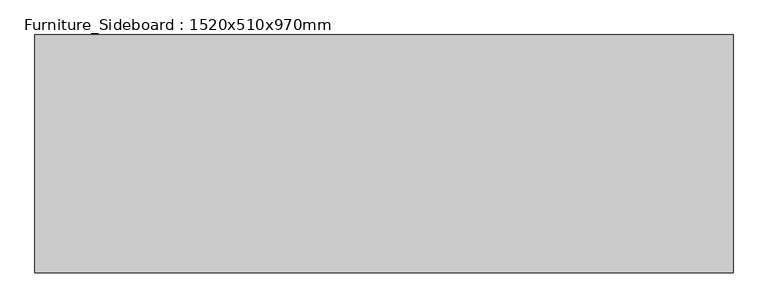
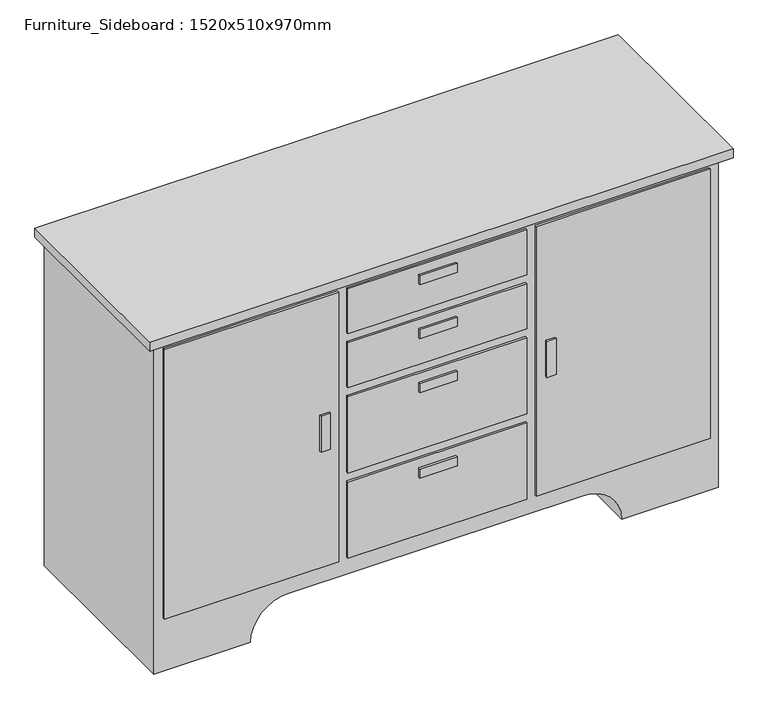
"""IFC4 building model written with IfcOpenShell, lengths in millimetres: furniture geometry, Furniture_Sideboard : 1520x510x970mm."""

from ifc_helpers import new_model, si_unit, point, frame, frame_2d, origin, place, context, project, spatial, polyline, circle_curve, trimmed, segment, composite_curve, outline, extrude, source, transform, mapped, element, save


def furniture_sideboard_1520x510x970mm_787d3fa7(model_context):
    return source(origin(), model_context, "Body", "SweptSolid", [
        extrude(outline(composite_curve([segment(polyline([(0.3974948, 465.4067402), (944.9401786, 465.4067402), (944.9401786, -1054.5932598), (0.3401786, -1054.5932598), (0.3401786, -794.7676781)]), True, "CONTINUOUS"), segment(trimmed(circle_curve(frame_2d((0.3401786, -691.2410879)), 103.5265902), [point((0.3401786, -794.7676781))], [point((103.8667688, -691.2410879))], True, "CARTESIAN"), True, "CONTINUOUS"), segment(polyline([(103.8667688, -691.2410879), (103.8667688, 102.4734638)]), True, "CONTINUOUS"), segment(trimmed(circle_curve(frame_2d((0.3974948, 102.4734638)), 103.469274), [point((103.8667688, 102.4734638))], [point((0.3974948, 205.9427378))], True, "CARTESIAN"), True, "CONTINUOUS"), segment(polyline([(0.3974948, 205.9427378), (0.3974948, 465.4067402)]), True, "CONTINUOUS")], self_intersect=False)), frame((0.0, -618.1629541, 0.0), z_axis=(0.0, 1.0, 0.0), x_axis=(0.0, 0.0, 1.0)), (0.0, 0.0, 1.0), 510.0),
        extrude(outline(polyline([(490.8067402, -643.5629541), (-1079.9932598, -643.5629541), (-1079.9932598, -108.1629541), (490.8067402, -108.1629541), (490.8067402, -643.5629541)])), frame((0.0, 0.0, 944.9401786), z_axis=(0.0, 0.0, 1.0), x_axis=(1.0, 0.0, 0.0)), (0.0, 0.0, 1.0), 25.4),
        extrude(outline(polyline([(-560.6265932, -624.5129541), (-1029.1932598, -624.5129541), (-1029.1932598, -618.1629541), (-560.6265932, -618.1629541), (-560.6265932, -624.5129541)])), frame((0.0, 0.0, 152.4), z_axis=(0.0, 0.0, 1.0), x_axis=(1.0, 0.0, 0.0)), (0.0, 0.0, 1.0), 767.1401786),
        extrude(outline(polyline([(440.0067402, -624.5129541), (-28.5599265, -624.5129541), (-28.5599265, -618.1629541), (440.0067402, -618.1629541), (440.0067402, -624.5129541)])), frame((0.0, 0.0, 152.4), z_axis=(0.0, 0.0, 1.0), x_axis=(1.0, 0.0, 0.0)), (0.0, 0.0, 1.0), 767.1401786),
        extrude(outline(polyline([(-53.9599265, -624.5129541), (-535.2265932, -624.5129541), (-535.2265932, -618.1629541), (-53.9599265, -618.1629541), (-53.9599265, -624.5129541)])), frame((0.0, 0.0, 791.5121429), z_axis=(0.0, 0.0, 1.0), x_axis=(1.0, 0.0, 0.0)), (0.0, 0.0, 1.0), 128.0280357),
        extrude(outline(polyline([(-53.9599265, -624.5129541), (-535.2265932, -624.5129541), (-535.2265932, -618.1629541), (-53.9599265, -618.1629541), (-53.9599265, -624.5129541)])), frame((0.0, 0.0, 638.0841071), z_axis=(0.0, 0.0, 1.0), x_axis=(1.0, 0.0, 0.0)), (0.0, 0.0, 1.0), 128.0280357),
        extrude(outline(polyline([(-53.9599265, -624.5129541), (-535.2265932, -624.5129541), (-535.2265932, -618.1629541), (-53.9599265, -618.1629541), (-53.9599265, -624.5129541)])), frame((0.0, 0.0, 395.2420536), z_axis=(0.0, 0.0, 1.0), x_axis=(1.0, 0.0, 0.0)), (0.0, 0.0, 1.0), 217.4420536),
        extrude(outline(polyline([(-53.9599265, -624.5129541), (-535.2265932, -624.5129541), (-535.2265932, -618.1629541), (-53.9599265, -618.1629541), (-53.9599265, -624.5129541)])), frame((0.0, 0.0, 152.4), z_axis=(0.0, 0.0, 1.0), x_axis=(1.0, 0.0, 0.0)), (0.0, 0.0, 1.0), 217.4420536),
        extrude(outline(polyline([(-586.0265932, -630.8629541), (-611.4265932, -630.8629541), (-611.4265932, -624.5129541), (-586.0265932, -624.5129541), (-586.0265932, -630.8629541)])), frame((0.0, 0.0, 484.758125), z_axis=(0.0, 0.0, 1.0), x_axis=(1.0, 0.0, 0.0)), (0.0, 0.0, 1.0), 102.56),
        extrude(outline(polyline([(-244.5230145, -630.8629541), (-346.0702491, -630.8629541), (-346.0702491, -624.5129541), (-244.5230145, -624.5129541), (-244.5230145, -630.8629541)])), frame((0.0, 0.0, 868.7401786), z_axis=(0.0, 0.0, 1.0), x_axis=(1.0, 0.0, 0.0)), (0.0, 0.0, 1.0), 25.4),
        extrude(outline(polyline([(-244.5230145, -630.8629541), (-346.0702491, -630.8629541), (-346.0702491, -624.5129541), (-244.5230145, -624.5129541), (-244.5230145, -630.8629541)])), frame((0.0, 0.0, 715.3121429), z_axis=(0.0, 0.0, 1.0), x_axis=(1.0, 0.0, 0.0)), (0.0, 0.0, 1.0), 25.4),
        extrude(outline(polyline([(-244.5230145, -630.8629541), (-346.0702491, -630.8629541), (-346.0702491, -624.5129541), (-244.5230145, -624.5129541), (-244.5230145, -630.8629541)])), frame((0.0, 0.0, 561.918125), z_axis=(0.0, 0.0, 1.0), x_axis=(1.0, 0.0, 0.0)), (0.0, 0.0, 1.0), 25.4),
        extrude(outline(polyline([(-244.5230145, -630.8629541), (-346.0702491, -630.8629541), (-346.0702491, -624.5129541), (-244.5230145, -624.5129541), (-244.5230145, -630.8629541)])), frame((0.0, 0.0, 318.5620536), z_axis=(0.0, 0.0, 1.0), x_axis=(1.0, 0.0, 0.0)), (0.0, 0.0, 1.0), 25.88),
        extrude(outline(polyline([(22.2400735, -630.8629541), (-3.1599265, -630.8629541), (-3.1599265, -624.5129541), (22.2400735, -624.5129541), (22.2400735, -630.8629541)])), frame((0.0, 0.0, 484.758125), z_axis=(0.0, 0.0, 1.0), x_axis=(1.0, 0.0, 0.0)), (0.0, 0.0, 1.0), 102.56),
    ])


if __name__ == "__main__":
    model = new_model("IFC4")
    model_context = context("Model", 3, world=origin())
    ifc_project = project(units=[si_unit("LENGTHUNIT", "METRE", prefix="MILLI")], contexts=[model_context])
    site = spatial("IfcSite", under=ifc_project)
    building = spatial("IfcBuilding", under=site)
    placement = place(None, origin())
    furniture_sideboard_1520x510x970mm_shape = furniture_sideboard_1520x510x970mm_787d3fa7(model_context)
    element("IfcFurniture", 1, ObjectType="Furniture_Sideboard : 1520x510x970mm", at=placement, inside=building, context=model_context, shape_type="MappedRepresentation", body=[
        mapped(furniture_sideboard_1520x510x970mm_shape, transform((0.0, 0.0, 0.0), x_axis=(1.0, 0.0, 0.0), y_axis=(0.0, 1.0, 0.0), z_axis=(0.0, 0.0, 1.0))),
    ])
    save(model, "model.ifc")

# Revit data of these elements
# Type "Furniture_Sideboard : 1520x510x970mm"
#   Keynote = "N"
#   Depth = 1' - 8.07874"
#   Height = 3' - 2.18898"
#   Width = 4' - 11.84252"
#   Material = Wood - Cherry
#   Default Elevation = 0
#   Assembly Code = ""
# Element 1 (IfcFurniture, "Furniture_Sideboard : 1520x510x970mm")
#   Materials on its faces: "Wood - Cherry"
# Materials
#   "Wood - Cherry": class "Wood", colour RGB 212 157 97, transparency 0
